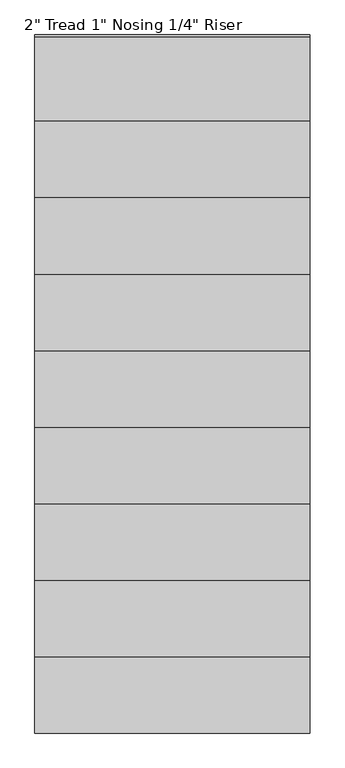
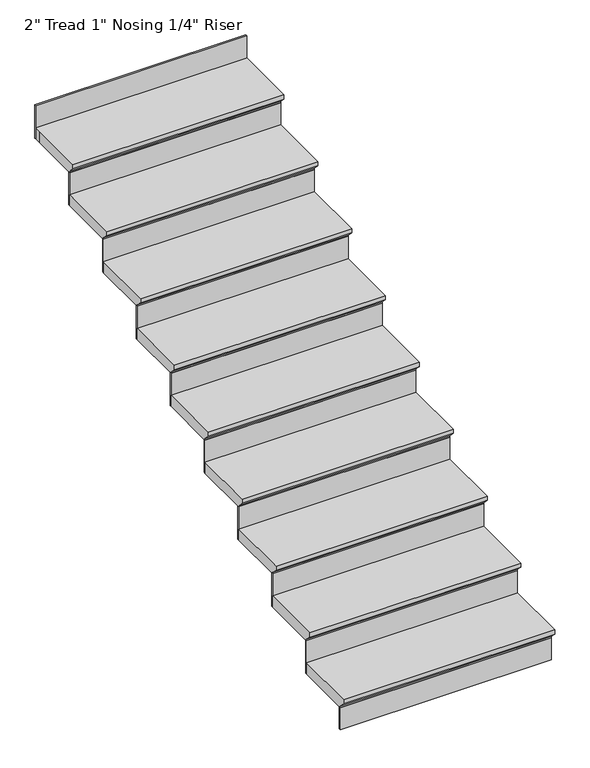
"""IFC4 building model written with IfcOpenShell, lengths in millimetres: stair flight geometry."""

from ifc_helpers import new_model, si_unit, origin, place, context, project, spatial, faceted_brep, source, transform, mapped, element, save


def stair_flight_63be9a33(model_context):
    return source(origin(), model_context, "Body", "Brep", [
        faceted_brep([(-9627.8771954, -4957.4727897, 3486.15), (-9627.8771954, -4957.4727897, 3505.2), (-10542.2771954, -4957.4727897, 3505.2), (-10542.2771954, -4957.4727897, 3486.15), (-9627.8771954, -4932.0727897, 3460.75), (-10542.2771954, -4932.0727897, 3460.75), (-9627.8771954, -4678.0727897, 3505.2), (-10542.2771954, -4678.0727897, 3505.2), (-10542.2771954, -4932.0727897, 3454.4), (-10542.2771954, -4678.0727897, 3454.4), (-9627.8771954, -4678.0727897, 3454.4), (-9627.8771954, -4932.0727897, 3454.4)], [[[0, 1, 2, 3]], [[4, 0, 3, 5]], [[2, 1, 6, 7]], [[8, 9, 10, 11]], [[2, 7, 9, 8, 5, 3]], [[8, 11, 4, 5]], [[6, 1, 0, 4, 11, 10]], [[7, 6, 10, 9]]]),
        faceted_brep([(-9627.8771954, -4932.0727897, 3454.4), (-9627.8771954, -4932.0727897, 3352.8), (-9627.8771954, -4925.7227897, 3352.8), (-9627.8771954, -4925.7227897, 3454.4), (-10542.2771954, -4932.0727897, 3454.4), (-10542.2771954, -4925.7227897, 3454.4), (-10542.2771954, -4925.7227897, 3352.8), (-10542.2771954, -4932.0727897, 3352.8)], [[[0, 1, 2, 3]], [[4, 5, 6, 7]], [[1, 0, 4, 7]], [[2, 1, 7, 6]], [[3, 2, 6, 5]], [[0, 3, 5, 4]]]),
        faceted_brep([(-9627.8771954, -4678.0727897, 3606.8), (-9627.8771954, -4678.0727897, 3454.4), (-9627.8771954, -4671.7227897, 3454.4), (-9627.8771954, -4671.7227897, 3606.8), (-10542.2771954, -4678.0727897, 3606.8), (-10542.2771954, -4671.7227897, 3606.8), (-10542.2771954, -4671.7227897, 3454.4), (-10542.2771954, -4678.0727897, 3454.4)], [[[0, 1, 2, 3]], [[4, 5, 6, 7]], [[1, 0, 4, 7]], [[2, 1, 7, 6]], [[3, 2, 6, 5]], [[0, 3, 5, 4]]]),
        faceted_brep([(-10542.2771954, -4703.4727897, 3657.6), (-9627.8771954, -4703.4727897, 3657.6), (-9627.8771954, -4424.0727897, 3657.6), (-10542.2771954, -4424.0727897, 3657.6), (-10542.2771954, -4678.0727897, 3606.8), (-10542.2771954, -4424.0727897, 3606.8), (-9627.8771954, -4424.0727897, 3606.8), (-9627.8771954, -4678.0727897, 3606.8), (-10542.2771954, -4678.0727897, 3613.15), (-10542.2771954, -4703.4727897, 3638.55), (-9627.8771954, -4678.0727897, 3613.15), (-9627.8771954, -4703.4727897, 3638.55)], [[[0, 1, 2, 3]], [[4, 5, 6, 7]], [[0, 3, 5, 4, 8, 9]], [[4, 7, 10, 8]], [[2, 1, 11, 10, 7, 6]], [[3, 2, 6, 5]], [[11, 1, 0, 9]], [[10, 11, 9, 8]]]),
        faceted_brep([(-9627.8771954, -4424.0727897, 3759.2), (-9627.8771954, -4424.0727897, 3606.8), (-9627.8771954, -4417.7227897, 3606.8), (-9627.8771954, -4417.7227897, 3759.2), (-10542.2771954, -4424.0727897, 3759.2), (-10542.2771954, -4417.7227897, 3759.2), (-10542.2771954, -4417.7227897, 3606.8), (-10542.2771954, -4424.0727897, 3606.8)], [[[0, 1, 2, 3]], [[4, 5, 6, 7]], [[1, 0, 4, 7]], [[2, 1, 7, 6]], [[3, 2, 6, 5]], [[0, 3, 5, 4]]]),
        faceted_brep([(-10542.2771954, -4449.4727897, 3810.0), (-9627.8771954, -4449.4727897, 3810.0), (-9627.8771954, -4170.0727897, 3810.0), (-10542.2771954, -4170.0727897, 3810.0), (-10542.2771954, -4424.0727897, 3759.2), (-10542.2771954, -4170.0727897, 3759.2), (-9627.8771954, -4170.0727897, 3759.2), (-9627.8771954, -4424.0727897, 3759.2), (-10542.2771954, -4424.0727897, 3765.55), (-10542.2771954, -4449.4727897, 3790.95), (-9627.8771954, -4424.0727897, 3765.55), (-9627.8771954, -4449.4727897, 3790.95)], [[[0, 1, 2, 3]], [[4, 5, 6, 7]], [[0, 3, 5, 4, 8, 9]], [[4, 7, 10, 8]], [[2, 1, 11, 10, 7, 6]], [[3, 2, 6, 5]], [[11, 1, 0, 9]], [[10, 11, 9, 8]]]),
        faceted_brep([(-9627.8771954, -4170.0727897, 3911.6), (-9627.8771954, -4170.0727897, 3759.2), (-9627.8771954, -4163.7227897, 3759.2), (-9627.8771954, -4163.7227897, 3911.6), (-10542.2771954, -4170.0727897, 3911.6), (-10542.2771954, -4163.7227897, 3911.6), (-10542.2771954, -4163.7227897, 3759.2), (-10542.2771954, -4170.0727897, 3759.2)], [[[0, 1, 2, 3]], [[4, 5, 6, 7]], [[1, 0, 4, 7]], [[2, 1, 7, 6]], [[3, 2, 6, 5]], [[0, 3, 5, 4]]]),
        faceted_brep([(-10542.2771954, -4195.4727897, 3962.4), (-9627.8771954, -4195.4727897, 3962.4), (-9627.8771954, -3916.0727897, 3962.4), (-10542.2771954, -3916.0727897, 3962.4), (-10542.2771954, -4170.0727897, 3911.6), (-10542.2771954, -3916.0727897, 3911.6), (-9627.8771954, -3916.0727897, 3911.6), (-9627.8771954, -4170.0727897, 3911.6), (-10542.2771954, -4170.0727897, 3917.95), (-10542.2771954, -4195.4727897, 3943.35), (-9627.8771954, -4170.0727897, 3917.95), (-9627.8771954, -4195.4727897, 3943.35)], [[[0, 1, 2, 3]], [[4, 5, 6, 7]], [[0, 3, 5, 4, 8, 9]], [[4, 7, 10, 8]], [[2, 1, 11, 10, 7, 6]], [[3, 2, 6, 5]], [[11, 1, 0, 9]], [[10, 11, 9, 8]]]),
        faceted_brep([(-9627.8771954, -3916.0727897, 4064.0), (-9627.8771954, -3916.0727897, 3911.6), (-9627.8771954, -3909.7227897, 3911.6), (-9627.8771954, -3909.7227897, 4064.0), (-10542.2771954, -3916.0727897, 4064.0), (-10542.2771954, -3909.7227897, 4064.0), (-10542.2771954, -3909.7227897, 3911.6), (-10542.2771954, -3916.0727897, 3911.6)], [[[0, 1, 2, 3]], [[4, 5, 6, 7]], [[1, 0, 4, 7]], [[2, 1, 7, 6]], [[3, 2, 6, 5]], [[0, 3, 5, 4]]]),
        faceted_brep([(-10542.2771954, -3941.4727897, 4114.8), (-9627.8771954, -3941.4727897, 4114.8), (-9627.8771954, -3662.0727897, 4114.8), (-10542.2771954, -3662.0727897, 4114.8), (-10542.2771954, -3916.0727897, 4064.0), (-10542.2771954, -3662.0727897, 4064.0), (-9627.8771954, -3662.0727897, 4064.0), (-9627.8771954, -3916.0727897, 4064.0), (-10542.2771954, -3916.0727897, 4070.35), (-10542.2771954, -3941.4727897, 4095.75), (-9627.8771954, -3916.0727897, 4070.35), (-9627.8771954, -3941.4727897, 4095.75)], [[[0, 1, 2, 3]], [[4, 5, 6, 7]], [[0, 3, 5, 4, 8, 9]], [[4, 7, 10, 8]], [[2, 1, 11, 10, 7, 6]], [[3, 2, 6, 5]], [[11, 1, 0, 9]], [[10, 11, 9, 8]]]),
        faceted_brep([(-9627.8771954, -3662.0727897, 4216.4), (-9627.8771954, -3662.0727897, 4064.0), (-9627.8771954, -3655.7227897, 4064.0), (-9627.8771954, -3655.7227897, 4216.4), (-10542.2771954, -3662.0727897, 4216.4), (-10542.2771954, -3655.7227897, 4216.4), (-10542.2771954, -3655.7227897, 4064.0), (-10542.2771954, -3662.0727897, 4064.0)], [[[0, 1, 2, 3]], [[4, 5, 6, 7]], [[1, 0, 4, 7]], [[2, 1, 7, 6]], [[3, 2, 6, 5]], [[0, 3, 5, 4]]]),
        faceted_brep([(-10542.2771954, -3687.4727897, 4267.2), (-9627.8771954, -3687.4727897, 4267.2), (-9627.8771954, -3408.0727897, 4267.2), (-10542.2771954, -3408.0727897, 4267.2), (-10542.2771954, -3662.0727897, 4216.4), (-10542.2771954, -3408.0727897, 4216.4), (-9627.8771954, -3408.0727897, 4216.4), (-9627.8771954, -3662.0727897, 4216.4), (-10542.2771954, -3662.0727897, 4222.75), (-10542.2771954, -3687.4727897, 4248.15), (-9627.8771954, -3662.0727897, 4222.75), (-9627.8771954, -3687.4727897, 4248.15)], [[[0, 1, 2, 3]], [[4, 5, 6, 7]], [[0, 3, 5, 4, 8, 9]], [[4, 7, 10, 8]], [[2, 1, 11, 10, 7, 6]], [[3, 2, 6, 5]], [[11, 1, 0, 9]], [[10, 11, 9, 8]]]),
        faceted_brep([(-9627.8771954, -3408.0727897, 4368.8), (-9627.8771954, -3408.0727897, 4216.4), (-9627.8771954, -3401.7227897, 4216.4), (-9627.8771954, -3401.7227897, 4368.8), (-10542.2771954, -3408.0727897, 4368.8), (-10542.2771954, -3401.7227897, 4368.8), (-10542.2771954, -3401.7227897, 4216.4), (-10542.2771954, -3408.0727897, 4216.4)], [[[0, 1, 2, 3]], [[4, 5, 6, 7]], [[1, 0, 4, 7]], [[2, 1, 7, 6]], [[3, 2, 6, 5]], [[0, 3, 5, 4]]]),
        faceted_brep([(-10542.2771954, -3433.4727897, 4419.6), (-9627.8771954, -3433.4727897, 4419.6), (-9627.8771954, -3154.0727897, 4419.6), (-10542.2771954, -3154.0727897, 4419.6), (-10542.2771954, -3408.0727897, 4368.8), (-10542.2771954, -3154.0727897, 4368.8), (-9627.8771954, -3154.0727897, 4368.8), (-9627.8771954, -3408.0727897, 4368.8), (-10542.2771954, -3408.0727897, 4375.15), (-10542.2771954, -3433.4727897, 4400.55), (-9627.8771954, -3408.0727897, 4375.15), (-9627.8771954, -3433.4727897, 4400.55)], [[[0, 1, 2, 3]], [[4, 5, 6, 7]], [[0, 3, 5, 4, 8, 9]], [[4, 7, 10, 8]], [[2, 1, 11, 10, 7, 6]], [[3, 2, 6, 5]], [[11, 1, 0, 9]], [[10, 11, 9, 8]]]),
        faceted_brep([(-9627.8771954, -3154.0727897, 4521.2), (-9627.8771954, -3154.0727897, 4368.8), (-9627.8771954, -3147.7227897, 4368.8), (-9627.8771954, -3147.7227897, 4521.2), (-10542.2771954, -3154.0727897, 4521.2), (-10542.2771954, -3147.7227897, 4521.2), (-10542.2771954, -3147.7227897, 4368.8), (-10542.2771954, -3154.0727897, 4368.8)], [[[0, 1, 2, 3]], [[4, 5, 6, 7]], [[1, 0, 4, 7]], [[2, 1, 7, 6]], [[3, 2, 6, 5]], [[0, 3, 5, 4]]]),
        faceted_brep([(-10542.2771954, -3179.4727897, 4572.0), (-9627.8771954, -3179.4727897, 4572.0), (-9627.8771954, -2900.0727897, 4572.0), (-10542.2771954, -2900.0727897, 4572.0), (-10542.2771954, -3154.0727897, 4521.2), (-10542.2771954, -2900.0727897, 4521.2), (-9627.8771954, -2900.0727897, 4521.2), (-9627.8771954, -3154.0727897, 4521.2), (-10542.2771954, -3154.0727897, 4527.55), (-10542.2771954, -3179.4727897, 4552.95), (-9627.8771954, -3154.0727897, 4527.55), (-9627.8771954, -3179.4727897, 4552.95)], [[[0, 1, 2, 3]], [[4, 5, 6, 7]], [[0, 3, 5, 4, 8, 9]], [[4, 7, 10, 8]], [[2, 1, 11, 10, 7, 6]], [[3, 2, 6, 5]], [[11, 1, 0, 9]], [[10, 11, 9, 8]]]),
        faceted_brep([(-9627.8771954, -2646.0727897, 4826.0), (-9627.8771954, -2646.0727897, 4673.6), (-9627.8771954, -2639.7227897, 4673.6), (-9627.8771954, -2639.7227897, 4826.0), (-10542.2771954, -2646.0727897, 4826.0), (-10542.2771954, -2639.7227897, 4826.0), (-10542.2771954, -2639.7227897, 4673.6), (-10542.2771954, -2646.0727897, 4673.6)], [[[0, 1, 2, 3]], [[4, 5, 6, 7]], [[1, 0, 4, 7]], [[2, 1, 7, 6]], [[3, 2, 6, 5]], [[0, 3, 5, 4]]]),
        faceted_brep([(-9627.8771954, -2900.0727897, 4673.6), (-9627.8771954, -2900.0727897, 4521.2), (-9627.8771954, -2893.7227897, 4521.2), (-9627.8771954, -2893.7227897, 4673.6), (-10542.2771954, -2900.0727897, 4673.6), (-10542.2771954, -2893.7227897, 4673.6), (-10542.2771954, -2893.7227897, 4521.2), (-10542.2771954, -2900.0727897, 4521.2)], [[[0, 1, 2, 3]], [[4, 5, 6, 7]], [[1, 0, 4, 7]], [[2, 1, 7, 6]], [[3, 2, 6, 5]], [[0, 3, 5, 4]]]),
        faceted_brep([(-10542.2771954, -2646.0727897, 4724.4), (-10542.2771954, -2671.4727897, 4724.4), (-10542.2771954, -2925.4727897, 4724.4), (-9627.8771954, -2925.4727897, 4724.4), (-9627.8771954, -2671.4727897, 4724.4), (-9627.8771954, -2646.0727897, 4724.4), (-10542.2771954, -2671.4727897, 4673.6), (-10542.2771954, -2646.0727897, 4673.6), (-9627.8771954, -2646.0727897, 4673.6), (-9627.8771954, -2671.4727897, 4673.6), (-9627.8771954, -2900.0727897, 4673.6), (-10542.2771954, -2900.0727897, 4673.6), (-10542.2771954, -2900.0727897, 4679.95), (-10542.2771954, -2925.4727897, 4705.35), (-9627.8771954, -2900.0727897, 4679.95), (-9627.8771954, -2925.4727897, 4705.35)], [[[0, 1, 2, 3, 4, 5]], [[6, 7, 8, 9, 10, 11]], [[1, 0, 7, 6]], [[2, 1, 6, 11, 12, 13]], [[11, 10, 14, 12]], [[4, 3, 15, 14, 10, 9]], [[5, 4, 9, 8]], [[0, 5, 8, 7]], [[15, 3, 2, 13]], [[14, 15, 13, 12]]]),
    ])


if __name__ == "__main__":
    model = new_model("IFC4")
    model_context = context("Model", 3, world=origin())
    ifc_project = project(units=[si_unit("LENGTHUNIT", "METRE", prefix="MILLI")], contexts=[model_context])
    site = spatial("IfcSite", under=ifc_project)
    building = spatial("IfcBuilding", under=site)
    placement = place(None, origin())
    stair_flight_shape = stair_flight_63be9a33(model_context)
    element("IfcStairFlight", 1, ObjectType="2\" Tread 1\" Nosing 1/4\" Riser", at=placement, inside=building, context=model_context, shape_type="MappedRepresentation", body=[
        mapped(stair_flight_shape, transform((0.0, 0.0, 0.0), x_axis=(1.0, 0.0, 0.0), y_axis=(0.0, 1.0, 0.0), z_axis=(0.0, 0.0, 1.0))),
    ])
    save(model, "model.ifc")
